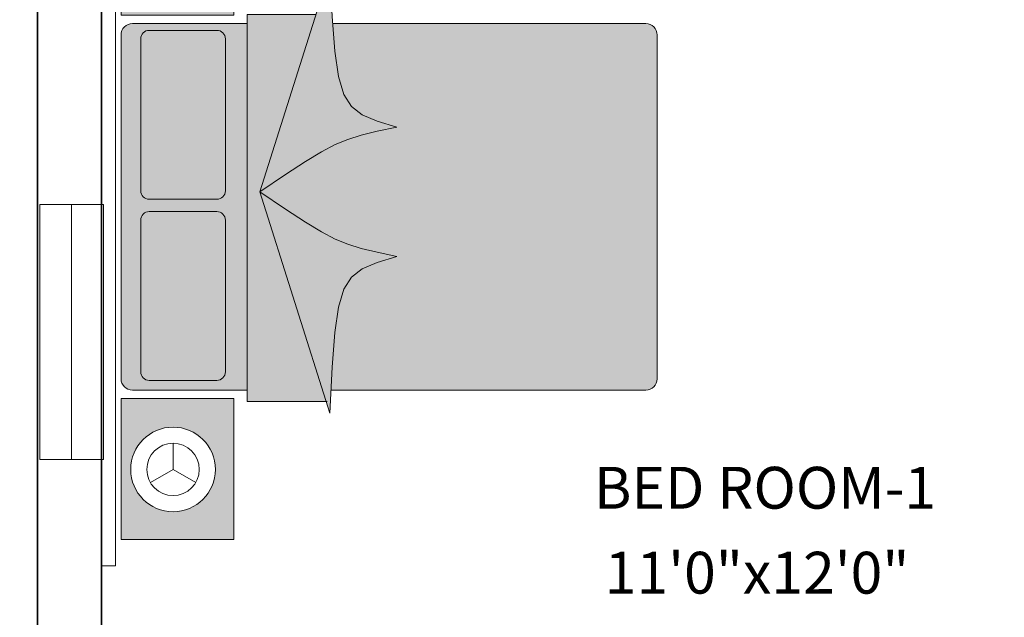
# Model space of a CAD drawing. Units: millimetres. Extents: x 27017497 to 27018854, y 7058029 to 7059154.
# Tile 44 of 91: x 27017611 to 27017750, y 7058472 to 7058557. Entities that reach past the tile are written whole.
import ezdxf

# ---------------------------------------------------------------- set-up
doc = ezdxf.new("R2010")
doc.units = ezdxf.units.MM
for name, color, linetype, lineweight in [('A-ANNO-DIMS', 2, 'Continuous', 18), ('A-AREA-IDEN', 7, 'Continuous', 18), ('A-FURN', 8, 'Continuous', 18), ('A-GLAZ', 4, 'Continuous', 18), ('A-WALL', 7, 'Continuous', 35)]:
    doc.layers.add(name, color=color, linetype=linetype, lineweight=lineweight)
doc.layers.add('A-FURN-PATT', color=177, linetype='Continuous', lineweight=13, true_color=0x293189)
doc.styles.get("Standard").update_dxf_attribs({"font": 'arial.ttf'})
doc.dimstyles.get("Standard").update_dxf_attribs({"dimtxt": 0.18, "dimasz": 0.18, "dimexe": 0.18, "dimexo": 0.0625, "dimgap": 0.09, "dimtad": 0, "dimtih": 1, "dimtoh": 1, "dimdec": 4, "dimzin": 0, "dimdsep": 46, "dimtxsty": 'Standard', "dimcen": 0.09, "dimadec": 0, "dimazin": 0, "dimtfac": 1, "dimtdec": 4, "dimtofl": 0, "dimtmove": 0, "dimatfit": 3, "dimfxl": 1, "dimtolj": 1, "dimtzin": 0, "dimarcsym": 0})

# ---------------------------------------------------------------- blocks, each defined once
blk = doc.blocks.new('CAMMAT')
for p, q in [((1.2731, 0), (-1.2731, 0)), ((1.2731, 0), (1.2731, -0.05)), ((-1.2731, 0), (-1.2731, -0.05)), ((1.2731, -0.05), (-1.2731, -0.05)), ((-1.18, -0.07), (-1.18, -0.47)), ((-1.18, -0.07), (-0.68, -0.07)), ((-0.68, -0.07), (-0.68, -0.47)), ((0.61, -0.07), (-0.61, -0.07)), ((0.68, -0.07), (0.68, -0.47)), ((0.68, -0.07), (1.18, -0.07)), ((1.18, -0.07), (1.18, -0.47)), ((-0.65, -0.11), (-0.65, -0.5169)), ((-0.0465, -0.1395), (-0.5852, -0.1395)), ((0.5962, -0.1395), (0.0574, -0.1395)), ((0.65, -0.11), (0.65, -0.5169)), ((-0.931, -0.2541), (-0.9775, -0.1737)), ((-0.6152, -0.1695), (-0.6152, -0.4095)), ((-0.0165, -0.1695), (-0.0165, -0.4095)), ((0.0274, -0.1695), (0.0274, -0.4095)), ((0.6262, -0.1695), (0.6262, -0.4095)), ((0.9242, -0.2541), (0.8777, -0.1737)), ((-0.931, -0.2541), (-0.9775, -0.3346)), ((-0.931, -0.2541), (-0.8381, -0.2541)), ((0.9242, -0.2541), (0.8777, -0.3346)), ((0.9242, -0.2541), (1.0171, -0.2541)), ((-0.0465, -0.4395), (-0.5852, -0.4395)), ((0.5962, -0.4395), (0.0574, -0.4395)), ((-1.18, -0.47), (-0.68, -0.47)), ((0.68, -0.47), (1.18, -0.47)), ((-0.6904, -0.5169), (-0.6904, -0.8)), ((-0.6904, -0.5169), (0.6826, -0.5169)), ((0.6826, -0.5169), (0.6826, -0.7603)), ((0.0535, -0.5623), (-0.7312, -0.8093)), ((0.0535, -0.5623), (0.8382, -0.8093)), ((-0.65, -0.8139), (-0.65, -1.93)), ((0.65, -0.8204), (0.65, -1.93)), ((0.61, -1.97), (-0.61, -1.97))]:
    blk.add_line(p, q)
for points in [[(-0.1761, -1.0476), (-0.161, -0.9772), (-0.1474, -0.921), (-0.1326, -0.8732), (-0.1139, -0.8282), (-0.0886, -0.7803), (-0.0541, -0.7238), (-0.0076, -0.653), (0.0535, -0.5623)], [(0.2832, -1.0476), (0.2681, -0.9772), (0.2545, -0.921), (0.2396, -0.8732), (0.2209, -0.8282), (0.1957, -0.7803), (0.1611, -0.7238), (0.1147, -0.653), (0.0535, -0.5623)], [(-0.7312, -0.8093), (-0.5683, -0.8185), (-0.4451, -0.828), (-0.3552, -0.8406), (-0.2919, -0.8591), (-0.2489, -0.8862), (-0.2196, -0.9248), (-0.1975, -0.9777), (-0.1761, -1.0476)], [(0.8382, -0.8093), (0.6753, -0.8185), (0.5522, -0.828), (0.4622, -0.8406), (0.399, -0.8591), (0.356, -0.8862), (0.3267, -0.9248), (0.3046, -0.9777), (0.2832, -1.0476)]]:
    blk.add_lwpolyline(points)
for centre, radius in [((-0.931, -0.2541), 0.15), ((0.9242, -0.2541), 0.15), ((-0.931, -0.2541), 0.0929), ((0.9242, -0.2541), 0.0929)]:
    blk.add_circle(centre, radius)
for centre, radius, start, end in [((-0.61, -0.11), 0.04, 90, 180), ((0.61, -0.11), 0.04, 0, 90), ((-0.5852, -0.1695), 0.03, 90, 180), ((-0.0465, -0.1695), 0.03, 360, 90), ((0.0574, -0.1695), 0.03, 90, 180), ((0.5962, -0.1695), 0.03, 360, 90), ((-0.5852, -0.4095), 0.03, 180, 270), ((-0.0465, -0.4095), 0.03, 270, 360), ((0.0574, -0.4095), 0.03, 180, 270), ((0.5962, -0.4095), 0.03, 270, 360), ((-0.61, -1.93), 0.04, 180, 270), ((0.61, -1.93), 0.04, 270, 360)]:
    blk.add_arc(centre, radius, start, end)
blk = doc.blocks.new('WINDOW-SINGLE-LIGHT')
blk.add_lwpolyline([(36, 4.5), (36, 0), (0, 0), (0, 9), (36, 9), (36, 4.5), (0, 4.5)])
blk = doc.blocks.new('*D48')
at = {"layer": 'A-ANNO-DIMS', "color": 0, "lineweight": -2, "transparency": 16777216}
for p, q in [((27018463.5, 7058622.91), (27017497.54, 7058622.91)), ((27017497.72, 7058622.73), (27017497.72, 7058357.75)), ((27017497.72, 7058092.41), (27017497.72, 7058357.39)), ((27018555.13, 7058092.23), (27017497.54, 7058092.23))]:
    blk.add_line(p, q, dxfattribs=at)
at = {"layer": 'A-ANNO-DIMS', "color": 0, "transparency": 16777216}
for points in [[(27017497.69, 7058622.73), (27017497.75, 7058622.73), (27017497.72, 7058622.91)], [(27017497.69, 7058092.41), (27017497.75, 7058092.41), (27017497.72, 7058092.23)]]:
    blk.add_solid(points, dxfattribs=at)
at = {"layer": 'Defpoints', "color": 0, "transparency": 16777216}
for p in [(27018463.56, 7058622.91), (27017497.72, 7058092.23), (27018555.19, 7058092.23)]:
    blk.add_point(p, dxfattribs=at)
at = {"layer": 'A-ANNO-DIMS', "color": 0, "transparency": 16777216, "insert": (27017497.72, 7058357.57), "char_height": 0.18, "attachment_point": 5}
blk.add_mtext('\\A1;530.7', dxfattribs=at)

msp = doc.modelspace()

# ---------------------------------------------------------------- hatches: boundary and pattern name
at = {"layer": 'A-FURN-PATT'}
h = msp.add_hatch(color=256, dxfattribs=at)
h.dxf.hatch_style = 1
h.paths.add_polyline_path([(27017701.132, 7058554.502, 0.4142136), (27017699.539, 7058556.096), (27017655.346, 7058556.096), (27017655.646, 7058552.199), (27017656.148, 7058548.617), (27017656.883, 7058546.099), (27017657.965, 7058544.385), (27017659.503, 7058543.218), (27017661.609, 7058542.338), (27017664.394, 7058541.486), (27017661.59, 7058540.884), (27017659.349, 7058540.341), (27017657.446, 7058539.751), (27017655.654, 7058539.006), (27017653.746, 7058538), (27017651.496, 7058536.625), (27017648.677, 7058534.773), (27017645.063, 7058532.339), (27017648.677, 7058529.904), (27017651.496, 7058528.052), (27017653.746, 7058526.677), (27017655.654, 7058525.671), (27017657.446, 7058524.926), (27017659.349, 7058524.336), (27017661.59, 7058523.794), (27017664.394, 7058523.191), (27017661.609, 7058522.339), (27017659.503, 7058521.459), (27017657.965, 7058520.292), (27017656.883, 7058518.579), (27017656.148, 7058516.06), (27017655.646, 7058512.478), (27017655.268, 7058507.572), (27017655.084, 7058504.317), (27017699.539, 7058504.317, 0.4142136), (27017701.132, 7058505.91)])
h.paths.add_polyline_path([(27017652.949, 7058557.393), (27017643.257, 7058557.393), (27017643.257, 7058502.708), (27017654.39, 7058502.708), (27017645.063, 7058532.339)])
h.paths.add_polyline_path([(27017656.883, 7058546.099), (27017656.148, 7058548.617), (27017655.646, 7058552.199), (27017655.268, 7058557.105), (27017654.901, 7058563.593), (27017645.063, 7058532.339), (27017648.677, 7058534.773), (27017651.496, 7058536.625), (27017653.746, 7058538), (27017655.654, 7058539.006), (27017657.446, 7058539.751), (27017659.349, 7058540.341), (27017661.59, 7058540.884), (27017664.394, 7058541.486), (27017661.609, 7058542.338), (27017659.503, 7058543.218), (27017657.965, 7058544.385)])
h.paths.add_polyline_path([(27017659.503, 7058521.459), (27017661.609, 7058522.339), (27017664.394, 7058523.191), (27017661.59, 7058523.794), (27017659.349, 7058524.336), (27017657.446, 7058524.926), (27017655.654, 7058525.671), (27017653.746, 7058526.677), (27017651.496, 7058528.052), (27017648.677, 7058529.904), (27017645.063, 7058532.339), (27017654.39, 7058502.708), (27017654.901, 7058501.084), (27017655.268, 7058507.572), (27017655.646, 7058512.478), (27017656.148, 7058516.06), (27017656.883, 7058518.579), (27017657.965, 7058520.292)])
h.paths.add_polyline_path([(27017640.173, 7058553.952, 0.4142136), (27017638.978, 7058555.147), (27017629.419, 7058555.147, 0.4142136), (27017628.224, 7058553.952), (27017628.224, 7058532.493, 0.4142136), (27017629.419, 7058531.298), (27017638.978, 7058531.298, 0.4142136), (27017640.173, 7058532.493)], flags=0)
h.paths.add_polyline_path([(27017640.173, 7058528.356, 0.4142136), (27017638.978, 7058529.551), (27017629.419, 7058529.551, 0.4142136), (27017628.224, 7058528.356), (27017628.224, 7058506.896, 0.4142136), (27017629.419, 7058505.701), (27017638.978, 7058505.701, 0.4142136), (27017640.173, 7058506.896)], flags=16)
h.paths.add_polyline_path([(27017643.257, 7058556.096), (27017627.049, 7058556.096, 0.4142136), (27017625.455, 7058554.502), (27017625.455, 7058505.91, 0.4142136), (27017627.049, 7058504.317), (27017643.257, 7058504.317)])
h.paths.add_polyline_path([(27017638.978, 7058531.298), (27017629.419, 7058531.298, -0.4142136), (27017628.224, 7058532.493), (27017628.224, 7058553.952, -0.4142136), (27017629.419, 7058555.147), (27017638.978, 7058555.147, -0.4142136), (27017640.173, 7058553.952), (27017640.173, 7058532.493, -0.4142136)], flags=16)
h.paths.add_polyline_path([(27017640.173, 7058528.356), (27017640.173, 7058506.896, -0.4142136), (27017638.978, 7058505.701), (27017629.419, 7058505.701, -0.4142136), (27017628.224, 7058506.896), (27017628.224, 7058528.356, -0.4142136), (27017629.419, 7058529.551), (27017638.978, 7058529.551, -0.4142136)], flags=0)
h.paths.add_polyline_path([(27017641.387, 7058503.122), (27017625.455, 7058503.122), (27017625.455, 7058483.207), (27017641.387, 7058483.207)])
h.paths.add_polyline_path([(27017626.814, 7058493.123, -1), (27017638.763, 7058493.123, -1)], flags=16)
h.paths.add_polyline_path([(27017629.088, 7058493.123, -1), (27017636.488, 7058493.123, -1)], flags=0)
h.paths.add_polyline_path([(27017641.387, 7058577.205), (27017625.455, 7058577.205), (27017625.455, 7058557.29), (27017641.387, 7058557.29)])
h.paths.add_polyline_path([(27017626.814, 7058567.015, -1), (27017638.763, 7058567.015, -1)], flags=16)
h.paths.add_polyline_path([(27017629.088, 7058567.015, -1), (27017636.488, 7058567.015, -1)], flags=0)
h = msp.add_hatch(color=256, dxfattribs=at)
h.dxf.hatch_style = 1
h.paths.add_polyline_path([(27017640.173, 7058553.952, 0.4142136), (27017638.978, 7058555.147), (27017629.419, 7058555.147, 0.4142136), (27017628.224, 7058553.952), (27017628.224, 7058532.493, 0.4142136), (27017629.419, 7058531.298), (27017638.978, 7058531.298, 0.4142136), (27017640.173, 7058532.493)])
h.paths.add_polyline_path([(27017640.173, 7058528.356, 0.4142136), (27017638.978, 7058529.551), (27017629.419, 7058529.551, 0.4142136), (27017628.224, 7058528.356), (27017628.224, 7058506.896, 0.4142136), (27017629.419, 7058505.701), (27017638.978, 7058505.701, 0.4142136), (27017640.173, 7058506.896)])

# ---------------------------------------------------------------- linework, layer by layer
at = {"layer": 'A-WALL'}
for p, q in [((27017613.666, 7058589.912), (27017613.666, 7058437.098)), ((27017622.666, 7058580.912), (27017622.666, 7058436.912))]:
    msp.add_line(p, q, dxfattribs=at)

# ---------------------------------------------------------------- block references
at = {"layer": 'A-FURN', "xscale": 39.82996475819422, "yscale": 39.82996475819422, "zscale": 39.82996475819422, "rotation": 89.99999999999999}
msp.add_blockref('CAMMAT', (27017622.667, 7058530.206), dxfattribs=at)
at = {"layer": 'A-GLAZ', "rotation": 270}
msp.add_blockref('WINDOW-SINGLE-LIGHT', (27017613.961, 7058530.539), dxfattribs=at)

# ---------------------------------------------------------------- texts
at = {"layer": 'A-ANNO-DIMS'}
msp.add_text('11\'0"x12\'0"', height=5.91176, dxfattribs=at).set_placement((27017693.745, 7058475.579))
at = {"layer": 'A-AREA-IDEN'}
msp.add_text('BED ROOM-1', height=5.9118, dxfattribs=at).set_placement((27017692.21, 7058487.577))

# ---------------------------------------------------------------- dimensions: what is measured, and where the dimension line sits
at = {"layer": 'A-ANNO-DIMS'}
dim = msp.add_linear_dim(base=(27017497.716, 7058092.23), p1=(27018463.561, 7058622.912), p2=(27018555.192, 7058092.23), angle=90, dimstyle='Standard', override={"dimdec": 1, "dimlfac": 1, "dimrnd": 0, "dimzin": 0, "dimdsep": 46, "dimlunit": 2}, dxfattribs=at)
dim.commit()
dim.dimension.update_dxf_attribs({"geometry": '*D48', "text_midpoint": (27017497.716, 7058357.571)})

doc.saveas('drawing.dxf')
